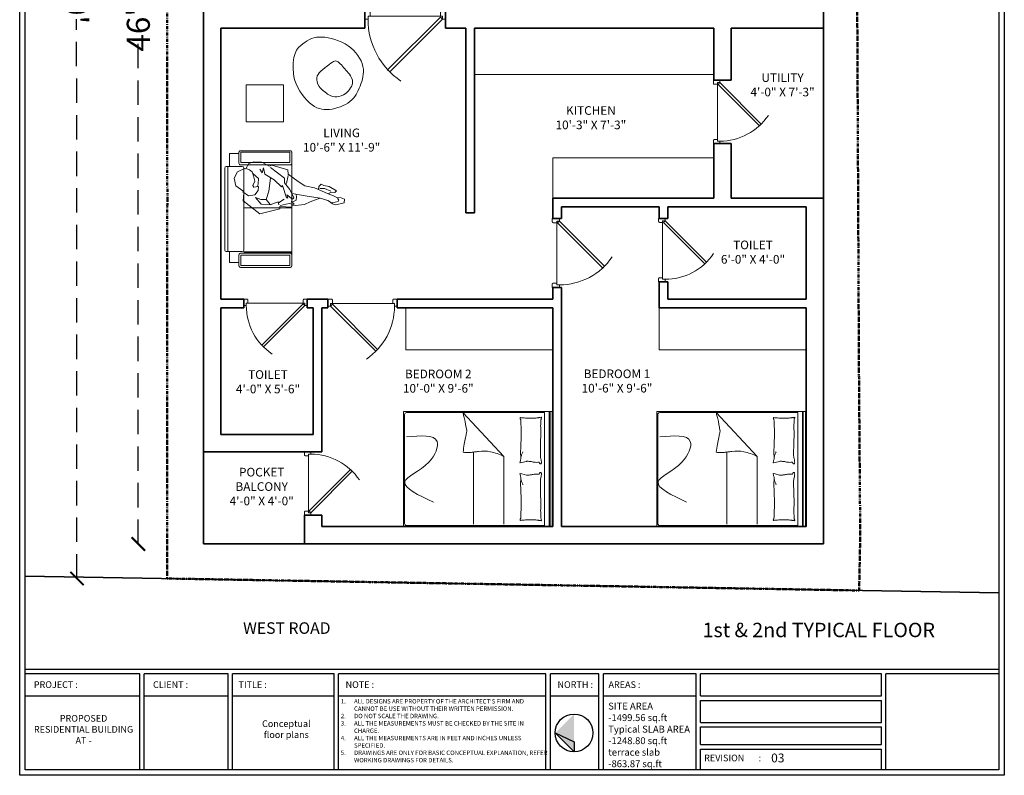
# Model space of a CAD drawing. Units: inches. Extents: x -16911 to -9621, y -48626 to -46270.
# Tile 2 of 20: x -16311 to -15799, y -47065 to -46672. Entities that reach past the tile are written whole.
import ezdxf

# ---------------------------------------------------------------- set-up
doc = ezdxf.new("R2010")
doc.units = ezdxf.units.IN
for name, pattern in [('DASHDOT', [1, 0.5, -0.25, 0, -0.25]), ('DASHED', [19.05, 12.7, -6.35]), ('DOT2', [3.175, 0, -3.175])]:
    doc.linetypes.add(name, pattern=pattern)
for name, color, linetype, lineweight in [('A-ANNO-DIMS', 2, 'Continuous', 13), ('A-ANNO-TEXT', 7, 'Continuous', 18), ('A-ANNO-TTLB', 7, 'Continuous', 25), ('A-AREA-IDEN', 3, 'Continuous', 18), ('A-DOOR', 4, 'Continuous', 18), ('A-FURN', 8, 'Continuous', 13), ('A-WALL', 7, 'Continuous', 35), ('C-PROP', 6, 'DASHDOT', 50), ('DOOR', 143, 'Continuous', 9), ('furniture', 35, 'Continuous', 15), ('Man', 8, 'Continuous', 5)]:
    doc.layers.add(name, color=color, linetype=linetype, lineweight=lineweight)
doc.styles.add('style9', font='swisscl.ttf', dxfattribs={"height": 12})
doc.dimstyles.new('Dim9', dxfattribs={"dimtxt": 10, "dimasz": 0.199219, "dimexe": 1, "dimexo": 0.5, "dimgap": 1, "dimtad": 0, "dimdec": 1, "dimzin": 0, "dimdsep": 46, "dimlunit": 4, "dimtxsty": 'style9', "dimblk": 'ARCHTICK', "dimcen": 0.09, "dimclrd": 256, "dimclrt": 256, "dimadec": 0, "dimazin": 0, "dimtfac": 1, "dimtdec": 1, "dimtix": 1, "dimtofl": 0, "dimtmove": 1, "dimatfit": 3, "dimfxl": 9, "dimtolj": 1, "dimtzin": 0, "dimlwd": -1, "dimarcsym": 0})

# ---------------------------------------------------------------- blocks, each defined once
blk = doc.blocks.new('Bipman02')
blk.add_lwpolyline([(0.5871, -0.067), (0.6175, -0.0496), (0.6523, -0.0539), (0.6697, -0.0376), (0.5958, 0.0069), (0.5437, 0.0156), (0.5164, 0.0297), (0.4959, 0.0069), (0.4915, -0.0235), (0.4524, -0.0061), (0.3568, 0.0113), (0.2917, 0.0548), (0.1917, 0.1287), (0.1874, 0.1722), (0.031, 0.2156), (0.0049, 0.2069), (-0.0689, 0.2461), (-0.1471, 0.2504), (-0.1949, 0.233), (-0.2253, 0.1808), (-0.2384, 0.1852), (-0.3079, 0.1504), (-0.3426, 0.0895), (-0.3253, 0.0113), (-0.2558, -0.0365), (-0.2471, -0.0583), (-0.2514, -0.1365), (-0.0863, -0.2626), (0.1092, -0.2148), (0.1092, -0.193), (0.2265, -0.1974), (0.2308, -0.1844), (0.3525, -0.1713), (0.409, -0.1452), (0.4872, -0.1148), (0.5089, -0.1104), (0.5828, -0.1322), (0.6088, -0.1496), (0.6295, -0.1636), (0.661, -0.1757), (0.7435, -0.1539), (0.7478, -0.1191), (0.7143, -0.1051), (0.674, -0.1017), (0.6392, -0.0844)], close=True)
for points in [[(-0.2558, -0.0452), (-0.1993, -0.0844), (-0.1385, -0.0757), (-0.1037, -0.0322), (-0.0994, 0.0069), (-0.1471, -0.0018), (-0.1558, 0.0156), (-0.1385, 0.0591), (-0.1515, 0.1113), (-0.1645, 0.1504), (-0.1906, 0.1722), (-0.2167, 0.1808)], [(-0.1558, 0.133), (-0.0994, 0.0852), (-0.1037, 0.033), (-0.1124, 0.0069)], [(-0.0863, 0.1765), (-0.0646, 0.1417), (-0.0516, 0.1895), (-0.0385, 0.1287), (0.0527, 0.0722), (0.1266, 0.0026), (0.1353, 0.0156), (0.1744, -0.1061), (0.1874, -0.1104), (0.1787, -0.0757), (0.2352, -0.1191), (0.2482, -0.1061), (0.2091, -0.0235), (0.157, 0.0417), (0.157, 0.0895), (0.018, 0.1939)], [(0.1917, 0.1156), (0.1744, 0.0374)], [(0.018, 0.0895), (0.0006, -0.0409), (-0.0255, -0.1235), (-0.0776, -0.1235), (-0.1298, -0.1017), (-0.0733, -0.167), (0.0136, -0.1757), (0.0918, -0.1452), (0.1005, -0.1757)], [(0.2699, -0.0757), (0.2743, -0.0974), (0.2699, -0.1278), (0.2439, -0.1409), (0.2222, -0.1452), (0.2482, -0.1626), (0.2482, -0.1713), (0.2004, -0.1626), (0.1135, -0.18)], [(0.2308, -0.0626), (0.3612, -0.0844), (0.5089, -0.1095)], [(0.4915, -0.0235), (0.5871, -0.067)], [(0.5045, -0.0148), (0.5523, -0.0148), (0.6132, -0.0409)], [(-0.0255, -0.1235), (0.0136, -0.1713)], [(0.0962, -0.1539), (0.1526, -0.1191)], [(0.6783, -0.1104), (0.6914, -0.1278), (0.687, -0.1409), (0.6566, -0.1496), (0.6088, -0.1539)]]:
    blk.add_lwpolyline(points)
blk = doc.blocks.new('erertety')
at = {"layer": 'furniture', "ltscale": 0.2}
for p, q in [((-17662.13, -45230.66), (-17662.13, -45176.69)), ((-17693.83, -45223.2), (-17693.83, -45184.43)), ((-17685.49, -45183.68), (-17693.08, -45183.68)), ((-17684.74, -45223.2), (-17684.74, -45184.43)), ((-17684.74, -45203.31), (-17662.13, -45203.31)), ((-17685.49, -45223.95), (-17693.08, -45223.95)), ((-17691.58, -45223.95), (-17691.58, -45229.1)), ((-17684.74, -45223.99), (-17662.13, -45223.99)), ((-17684.74, -45224.55), (-17662.13, -45224.55)), ((-17684.74, -45224.55), (-17662.13, -45224.55)), ((-17691.58, -45229.1), (-17687.09, -45229.1))]:
    blk.add_line(p, q, dxfattribs=at)
for points in [[(-17662.13, -45182.17), (-17662.13, -45176.97, 0.414214), (-17662.87, -45176.22), (-17686.34, -45176.22, 0.414214), (-17687.09, -45176.97), (-17687.09, -45182.17, 0.414214), (-17686.34, -45182.91), (-17662.87, -45182.91, 0.414214)], [(-17662.13, -45225.47), (-17662.13, -45230.66, -0.414214), (-17662.87, -45231.41), (-17686.34, -45231.41, -0.414214), (-17687.09, -45230.66), (-17687.09, -45225.47, -0.414214), (-17686.34, -45224.72), (-17662.87, -45224.72, -0.414214)]]:
    blk.add_lwpolyline(points, format="xyb", close=True, dxfattribs=at)
for points in [[(-17663.01, -45181.75), (-17663.01, -45176.82), (-17686.21, -45176.82), (-17686.21, -45181.75)], [(-17692.4, -45183.68), (-17692.4, -45223.95), (-17692.4, -45223.95), (-17692.4, -45183.68)], [(-17663.01, -45225.6), (-17663.01, -45230.53), (-17686.21, -45230.53), (-17686.21, -45225.6)]]:
    blk.add_lwpolyline(points, close=True, dxfattribs=at)
blk.add_lwpolyline([(-17687.09, -45177.54), (-17691.58, -45177.54), (-17691.58, -45183.68)], dxfattribs=at)
for centre, start, end in [((-17693.08, -45184.43), 90, 180), ((-17685.49, -45184.43), 0, 90), ((-17693.08, -45223.2), 180, 270), ((-17685.49, -45223.2), 270, 0)]:
    blk.add_arc(centre, 0.748, start, end, dxfattribs=at)
at = {"layer": 'furniture', "ltscale": 0.2, "xscale": 47.90818138957024, "yscale": 47.90818138957024, "zscale": 47.90818138957024}
blk.add_blockref('Bipman02', (-17673, -45193.44, 0), dxfattribs=at)
blk = doc.blocks.new('rthrty')
at = {"layer": 'furniture'}
blk.add_open_spline([(-17650.3, -45154.53), (-17651.97, -45142.9), (-17645.3, -45136.31), (-17637.11, -45132.37), (-17620.71, -45137.17), (-17612.47, -45149.45), (-17615.73, -45159.71), (-17619.67, -45168.02), (-17632.28, -45172.65), (-17641.84, -45170.43), (-17649.5, -45159.42), (-17650.3, -45154.53)], degree=3, dxfattribs=at)
at = {"layer": 'Man'}
blk.add_open_spline([(-17632.99, -45149.02), (-17629.89, -45146.6), (-17628, -45145.12), (-17623.29, -45151.15), (-17618.06, -45156.77), (-17623.15, -45164.08), (-17628.28, -45165.32), (-17631.61, -45164.6), (-17638.01, -45159.61), (-17638.81, -45154.69), (-17636.9, -45151.81), (-17632.99, -45149.02), (-17632.99, -45149.02)], degree=3, dxfattribs=at)
blk = doc.blocks.new('hjuyuiuyk')
at = {"layer": 'furniture'}
for p, q in [((-19327.49, -39738.98), (-19327.49, -39737.31)), ((-19327.49, -39737.31), (-19267.49, -39737.31, 0)), ((-19327.49, -39746.54), (-19327.49, -39737.31)), ((-19267.49, -39738.5), (-19327.49, -39738.5, 0)), ((-19327.49, -39738.5, 0), (-19327.49, -39814.72, 0)), ((-19327.49, -39738.5), (-19327.49, -39814.72)), ((-19267.49, -39738.5, 0), (-19327.49, -39738.5)), ((-19267.49, -39738.98, 0), (-19327.49, -39738.98)), ((-19267.49, -39737.31, 0), (-19267.49, -39738.98, 0)), ((-19267.49, -39746.54, 0), (-19267.49, -39737.31, 0)), ((-19267.49, -39814.72), (-19267.49, -39738.5)), ((-19267.49, -39814.72, 0), (-19267.49, -39738.5, 0)), ((-19268.1, -39741.33), (-19326.9, -39741.33)), ((-19326.9, -39741.33), (-19326.9, -39813.21)), ((-19268.1, -39813.21), (-19268.1, -39741.33)), ((-19300.88, -39753.22, 0), (-19301.49, -39750.81, 0)), ((-19300.67, -39754.09, 0), (-19300.88, -39753.22, 0)), ((-19295.19, -39754.09, 0), (-19294.97, -39753.22, 0)), ((-19294.97, -39753.22, 0), (-19294.37, -39750.81, 0)), ((-19304.07, -39762.52), (-19326.9, -39783.91)), ((-19304.07, -39762.52), (-19268.82, -39762.52)), ((-19268.82, -39778.34), (-19306.29, -39778.34)), ((-19326.9, -39813.21), (-19326.9, -39783.91)), ((-19327.49, -39814.72, 0), (-19267.49, -39814.72)), ((-19327.49, -39814.72), (-19267.49, -39814.72, 0)), ((-19269.1, -39814.21), (-19325.9, -39814.21)), ((-19325.9, -39814.21), (-19269.1, -39814.21))]:
    blk.add_line(p, q, dxfattribs=at)
for centre, radius, start, end in [((-19324.36, -39743.07, 0), 0.0997, 111.7883, 160.436), ((-19324.39, -39743.06, 0), 0.0676, 160.436, 281.8931), ((-19324.12, -39743.66, 0), 0.732, 94.3025, 111.7883), ((-19324.35, -39743.25, 0), 0.125, 21.9904, 101.8931), ((-19323.34, -39743.89, 0), 0.956, 158.579, 188.1335), ((-19317.18, -39743.01, 0), 7.17, 188.1335, 192.1095), ((-19324.65, -39743.37, 0), 0.455, 338.579, 21.9904), ((-19329.85, -39745.73, 0), 5.78, 7.6809, 12.1095), ((-19324.11, -39743.77, 0), 0.842, 59.3487, 94.3025), ((-19322.88, -39741.69, 0), 1.57, 239.3487, 264.7408), ((-19319.6, -39692.5, 0), 50.87, 266.1399, 268.6002), ((-19319.84, -39713.09, 0), 30.28, 268.0921, 271.2808), ((-19320.24, -39695.07, 0), 48.31, 271.2808, 273.4034), ((-19316.15, -39763.89, 0), 20.63, 90.1553, 93.4034), ((-19316.09, -39783.15, 0), 39.89, 86.9902, 90.1553), ((-19305.86, -39588.51, 0), 155.02, 266.9902, 268.5957), ((-19305.42, -39570.46, 0), 173.07, 268.5957, 270), ((-19305.42, -39718.38, 0), 25.15, 270, 273.6841), ((-19304.03, -39739.9, 0), 3.58, 273.6841, 287.1951), ((-19300.46, -39751.46, 0), 8.51, 98.4372, 107.1951), ((-19301.02, -39747.69, 0), 4.7, 90, 98.4372), ((-19301.12, -39743.14, 0), 0.997, 274.4002, 333.4195), ((-19315.3, -39745.68, 0), 14.34, 360, 6.2324), ((-19301.02, -39745.63, 0), 2.64, 78.7276, 90), ((-19300.58, -39743.42, 0), 0.383, 333.4195, 78.7276), ((-19295.28, -39743.42, 0), 0.383, 101.2724, 206.5805), ((-19294.73, -39743.14, 0), 0.997, 206.5805, 265.5998), ((-19294.84, -39745.63, 0), 2.64, 90, 101.2724), ((-19280.55, -39745.68, 0), 14.34, 173.7676, 180), ((-19294.84, -39747.69, 0), 4.7, 81.5628, 90), ((-19295.39, -39751.46, 0), 8.51, 72.8049, 81.5628), ((-19291.82, -39739.9, 0), 3.58, 252.8049, 266.3159), ((-19290.43, -39718.38, 0), 25.15, 266.3159, 270), ((-19290.43, -39570.46, 0), 173.07, 270, 271.4043), ((-19289.99, -39588.51, 0), 155.02, 271.4043, 273.0098), ((-19279.76, -39783.15, 0), 39.89, 89.8447, 93.0098), ((-19279.7, -39763.89, 0), 20.63, 86.5966, 89.8447), ((-19275.61, -39695.07, 0), 48.31, 266.5966, 268.7192), ((-19276.02, -39713.09, 0), 30.28, 268.7192, 271.9079), ((-19276.73, -39645.13, 0), 98.25, 271.0069, 272.7772), ((-19272.12, -39741.69, 0), 1.57, 275.2592, 300.6513), ((-19270.89, -39743.77, 0), 0.842, 85.6975, 120.6513), ((-19265.15, -39745.73, 0), 5.78, 167.8905, 172.3191), ((-19270.88, -39743.66, 0), 0.732, 68.2117, 85.6975), ((-19270.35, -39743.37, 0), 0.455, 158.0096, 201.421), ((-19277.82, -39743.01, 0), 7.17, 347.8905, 351.8665), ((-19270.65, -39743.25, 0), 0.125, 78.1069, 158.0096), ((-19271.66, -39743.89, 0), 0.956, 351.8665, 21.421), ((-19270.61, -39743.06, 0), 0.0676, 258.1069, 19.564), ((-19270.64, -39743.07, 0), 0.0997, 19.564, 68.2117), ((-19350.51, -39748.51, 0), 26.62, 3.3687, 7.6809), ((-19720.99, -39728.47, 0), 397.61, 356.4951, 356.945), ((-19363.7, -39747.54, 0), 39.81, 356.945, 358.3669), ((-19343.69, -39748.11, 0), 19.79, 358.3669, 3.3687), ((-19282.35, -39751.13, 0), 19.21, 171.9949, 177.3351), ((-19292.22, -39749.75, 0), 9.25, 167.8016, 171.9949), ((-19326.4, -39742.36, 0), 25.72, 347.8016, 350.3156), ((-19306.91, -39745.68, 0), 5.95, 350.3156, 360), ((-19288.94, -39745.68, 0), 5.95, 180, 189.6844), ((-19269.45, -39742.36, 0), 25.72, 189.6844, 192.1984), ((-19303.63, -39749.75, 0), 9.25, 8.0051, 12.1984), ((-19313.5, -39751.13, 0), 19.21, 2.6649, 8.0051), ((-19251.31, -39748.11, 0), 19.79, 176.6313, 181.6331), ((-19231.3, -39747.54, 0), 39.81, 181.6331, 183.055), ((-19244.49, -39748.51, 0), 26.62, 172.3191, 176.6313), ((-18874.01, -39728.47, 0), 397.61, 183.055, 183.5049), ((-19323.69, -39753.93, 0), 0.564, 170.0016, 196.6978), ((-19333.47, -39752.21, 0), 9.37, 350.0016, 356.4951), ((-19324.19, -39754.08, 0), 0.0385, 196.6978, 277.1204), ((-19324.51, -39751.59, 0), 2.55, 277.1204, 286.2212), ((-19324.42, -39751.9, 0), 2.23, 286.2212, 297.4439), ((-19322.81, -39754.99, 0), 1.25, 102.448, 117.4439), ((-19322.32, -39757.22, 0), 3.54, 93.574, 102.448), ((-19318.44, -39837.61, 0), 84.03, 90.9755, 92.7955), ((-19315.55, -39952.16, 0), 198.61, 89.4461, 91.2473), ((-19314.9, -39885.06, 0), 131.51, 87.2326, 89.4461), ((-19310.57, -39795.48, 0), 41.81, 85.4012, 87.2326), ((-19304.32, -39717.78, 0), 36.14, 265.4012, 267.3712), ((-19297.32, -39733.09, 0), 21.54, 244.6889, 246.5156), ((-19305.66, -39747.05, 0), 6.83, 267.3712, 281.4827), ((-19297.32, -39733.09, 0), 21.54, 246.5156, 248.3423), ((-19297.32, -39733.09, 0), 21.54, 248.3423, 250.572), ((-19297.32, -39733.09, 0), 21.54, 250.572, 252.8018), ((-19303.46, -39757.91, 0), 4.25, 83.5659, 101.4827), ((-19303.37, -39757.16, 0), 3.49, 72.6136, 83.5659), ((-19300.33, -39747.43, 0), 6.7, 252.6136, 260.5159), ((-19299.57, -39750.33, 0), 1.97, 177.3351, 194.0452), ((-19300.13, -39746.25, 0), 7.9, 260.5159, 265.9171), ((-19300.69, -39754.1, 0), 0.0267, 265.9171, 14.0449), ((-19295.16, -39754.1, 0), 0.0267, 165.9551, 274.0829), ((-19295.72, -39746.25, 0), 7.9, 274.0829, 279.4841), ((-19295.52, -39747.43, 0), 6.7, 279.4841, 287.3864), ((-19296.28, -39750.33, 0), 1.97, 345.9548, 2.6649), ((-19292.48, -39757.16, 0), 3.49, 96.4341, 107.3864), ((-19292.39, -39757.91, 0), 4.25, 78.5173, 96.4341), ((-19298.54, -39733.09, 0), 21.54, 287.1982, 289.428), ((-19290.19, -39747.05, 0), 6.83, 258.5173, 272.6288), ((-19298.54, -39733.09, 0), 21.54, 289.428, 291.6577), ((-19298.54, -39733.09, 0), 21.54, 291.6577, 293.4844), ((-19298.54, -39733.09, 0), 21.54, 293.4844, 295.3111), ((-19291.53, -39717.78, 0), 36.14, 272.6288, 274.5988), ((-19285.28, -39795.48, 0), 41.81, 92.7674, 94.5988), ((-19280.95, -39885.06, 0), 131.51, 90.5539, 92.7674), ((-19280.3, -39952.16, 0), 198.61, 88.7527, 90.5539), ((-19277.1, -39805.01, 0), 51.42, 86.426, 88.7527), ((-19274.68, -39799.75, 0), 46.07, 86.5575, 89.0171), ((-19272.19, -39754.99, 0), 1.25, 62.5561, 77.552), ((-19270.58, -39751.9, 0), 2.23, 242.5561, 253.7788), ((-19270.49, -39751.59, 0), 2.55, 253.7788, 262.8796), ((-19261.53, -39752.21, 0), 9.37, 183.5049, 189.9984), ((-19270.81, -39754.08, 0), 0.0385, 262.8796, 343.3022), ((-19271.31, -39753.93, 0), 0.564, 343.3022, 9.9984), ((-19279.47, -39774.89), 27.53, 153.3084, 168.7423), ((-19287.94, -39773.2), 18.89, 168.7423, 187.3994), ((-19242.78, -39767.34), 64.43, 187.3994, 189.2719), ((-19333.07, -39782.08), 27.05, 6.3817, 9.2719), ((-19321.79, -39780.82), 15.7, 359.2313, 6.3817), ((-19306.77, -39846.83), 66.07, 105.9352, 107.7364), ((-19318.41, -39806.06), 23.67, 102.9255, 105.9352), ((-19287.64, -39956.87), 177.57, 99.7243, 101.7196), ((-19317.24, -39783.9), 2.09, 82.2696, 100.7276), ((-19317.9, -39788.76), 6.99, 76.8096, 82.2696), ((-19295.64, -39693.77), 90.57, 256.8096, 258.3259), ((-19295.11, -39691.23), 93.17, 258.3259, 260.505), ((-19288.03, -39648.9), 136.08, 260.505, 262.308), ((-19336.71, -39780.62), 30.63, 354.1141, 359.2313), ((-19325.9, -39813.21), 1, 180, 270), ((-19269.1, -39813.21), 1, 270, 0)]:
    blk.add_arc(centre, radius, start, end, dxfattribs=at)
blk.add_open_spline([(-19280.24, -39799.21), (-19283.87, -39806.94), (-19290.73, -39821.55), (-19298.08, -39801.09), (-19315.85, -39793.47), (-19314.86, -39805.92), (-19314.29, -39813.13)], degree=3, knots=[0, 0, 0, 0, 18.167809, 34.338432, 45.972904, 61.997799, 61.997799, 61.997799, 61.997799], dxfattribs=at)
blk = doc.blocks.new('A$C1C9D3E54')
at = {"layer": 'DOOR'}
blk.add_line((18676.53, 5780.72), (18710.53, 5780.72), dxfattribs=at)
blk.add_lwpolyline([(18685.01, 5806.62), (18710.47, 5781.16), (18711.53, 5782.22), (18686.07, 5807.68), (18685.01, 5806.62)], dxfattribs=at)
blk.add_lwpolyline([(18674.03, 5778.22), (18676.03, 5778.22), (18674.03, 5778.22), (18674.03, 5782.22), (18675.53, 5782.22), (18675.53, 5780.72), (18676.53, 5780.72), (18676.53, 5778.72), (18676.41, 5778.72), (18676.41, 5778.6, -0.414214), (18676.16, 5778.35), (18676.03, 5778.35), (18676.03, 5778.22)], format="xyb", dxfattribs=at)
blk.add_lwpolyline([(18713.03, 5782.22), (18711.53, 5782.22), (18711.53, 5780.72), (18710.53, 5780.72), (18710.53, 5778.72), (18710.66, 5778.72), (18710.66, 5778.6, 0.414214), (18710.91, 5778.35), (18711.03, 5778.35), (18711.03, 5778.22), (18713.03, 5778.22), (18711.03, 5778.22), (18713.03, 5778.22), (18713.03, 5782.22)], format="xyb", close=True, dxfattribs=at)
blk.add_arc((18711.53, 5782.22), 36, 124.0336, 180, dxfattribs=at)
blk = doc.blocks.new('_ArchTick')
at = {"color": 0, "linetype": 'ByBlock', "const_width": 0.15}
blk.add_lwpolyline([(-0.5, -0.5), (0.5, 0.5)], dxfattribs=at)
blk = doc.blocks.new('*D58')
at = {"layer": 'A-ANNO-DIMS', "color": 0, "linetype": 'DOT2', "lineweight": -2, "transparency": 16777216}
for p, q in [((-16281.81, -46362.82), (-16283, -46362.82)), ((-16281.44, -46962.82), (-16282.63, -46962.82))]:
    blk.add_line(p, q, dxfattribs=at)
at = {"layer": 'A-ANNO-DIMS', "color": 0, "linetype": 'DASHED', "lineweight": 25, "transparency": 16777216}
for p, q in [((-16282, -46362.82), (-16281.82, -46653.98)), ((-16281.63, -46962.82), (-16281.81, -46671.67))]:
    blk.add_line(p, q, dxfattribs=at)
at = {"layer": 'Defpoints', "color": 0, "transparency": 16777216}
for p in [(-16282, -46362.82), (-16263.18, -46362.81), (-16262.82, -46962.81)]:
    blk.add_point(p, dxfattribs=at)
at = {"layer": 'A-ANNO-DIMS', "color": 0, "lineweight": 25, "transparency": 16777216, "xscale": 7, "yscale": 7, "zscale": 7}
for p, rotation in [((-16282, -46362.82), 90.0346840750536), ((-16281.63, -46962.82), 270.0346840750536)]:
    blk.add_blockref('_ArchTick', p, dxfattribs=dict(at, rotation=rotation))
at = {"layer": 'A-ANNO-DIMS', "color": 0, "transparency": 16777216, "insert": (-16281.81, -46662.82), "char_height": 12, "attachment_point": 5, "rotation": 270.0347, "style": 'style9'}
blk.add_mtext("\\A1;50'", dxfattribs=at)
blk = doc.blocks.new('*D60')
at = {"layer": 'A-ANNO-DIMS', "color": 0, "linetype": 'DOT2', "lineweight": -2, "transparency": 16777216}
for p, q in [((-16249.52, -46386.86), (-16250.71, -46386.86)), ((-16249.52, -46944.81), (-16250.71, -46944.81))]:
    blk.add_line(p, q, dxfattribs=at)
at = {"layer": 'A-ANNO-DIMS', "color": 0, "linetype": 'DASHED', "lineweight": 25, "transparency": 16777216}
for p, q in [((-16249.71, -46386.86), (-16249.71, -46648.2)), ((-16249.71, -46944.81), (-16249.71, -46683.47))]:
    blk.add_line(p, q, dxfattribs=at)
at = {"layer": 'Defpoints', "color": 0, "transparency": 16777216}
for p in [(-16215.78, -46386.86), (-16249.71, -46944.81), (-16215.78, -46944.81)]:
    blk.add_point(p, dxfattribs=at)
at = {"layer": 'A-ANNO-DIMS', "color": 0, "lineweight": 25, "transparency": 16777216, "xscale": 7, "yscale": 7, "zscale": 7}
for p, rotation in [((-16249.71, -46386.86), 90), ((-16249.71, -46944.81), 270)]:
    blk.add_blockref('_ArchTick', p, dxfattribs=dict(at, rotation=rotation))
at = {"layer": 'A-ANNO-DIMS', "color": 0, "transparency": 16777216, "insert": (-16249.71, -46665.83), "char_height": 12, "attachment_point": 5, "rotation": 90, "style": 'style9'}
blk.add_mtext('\\A1;46\'-6"', dxfattribs=at)
blk = doc.blocks.new('TITLE-BLOCK-A3')
blk.add_hatch(color=256).paths.add_polyline_path([(-16032.81, -47043.2), (-16022.97, -47033.35), (-16022.97, -47053.05)])
for p, q in [((-16311.44, -47065.27), (-16311.44, -46330.13)), ((-16308.66, -47062.49), (-16308.66, -46332.91)), ((-15801.86, -46332.91), (-15801.86, -47062.49)), ((-15799.07, -46330.13), (-15799.07, -47065.27)), ((-15801.86, -47010.14), (-16308.66, -47010.14)), ((-16248.93, -47012.43), (-16308.66, -47012.43)), ((-16248.93, -47062.49), (-16248.93, -47012.43)), ((-16202.98, -47012.43), (-16246.63, -47012.43)), ((-16246.63, -47062.49), (-16246.63, -47012.43)), ((-16202.98, -47062.49), (-16202.98, -47012.43)), ((-16147.85, -47012.43), (-16200.68, -47012.43)), ((-16200.68, -47062.49), (-16200.68, -47012.43)), ((-16147.85, -47062.49), (-16147.85, -47012.43)), ((-16037.57, -47012.43), (-16145.55, -47012.43)), ((-16145.55, -47062.49), (-16145.55, -47012.43)), ((-16037.57, -47062.49), (-16037.57, -47012.43)), ((-16010.01, -47012.43), (-16035.28, -47012.43)), ((-16035.28, -47062.49), (-16035.28, -47012.43)), ((-16010.01, -47062.49), (-16010.01, -47012.43)), ((-15959.47, -47012.43), (-16007.71, -47012.43)), ((-16007.71, -47062.49), (-16007.71, -47012.43)), ((-15959.47, -47062.49), (-15959.47, -47012.43)), ((-15862.98, -47012.43), (-15957.17, -47012.43)), ((-15957.17, -47023.95), (-15957.17, -47012.43)), ((-15862.98, -47023.95), (-15862.98, -47012.43)), ((-15801.86, -47012.43), (-15860.68, -47012.43)), ((-15860.68, -47062.49), (-15860.68, -47012.43)), ((-16308.66, -47023.95), (-16248.93, -47023.95)), ((-16246.63, -47023.95), (-16202.98, -47023.95)), ((-16200.68, -47023.95), (-16147.85, -47023.95)), ((-16145.55, -47023.95), (-16037.57, -47023.95)), ((-16035.28, -47023.95), (-16010.01, -47023.95)), ((-16007.71, -47023.95), (-15959.47, -47023.95)), ((-15957.17, -47023.95), (-15862.98, -47023.95)), ((-15957.17, -47037.77), (-15957.17, -47026.25)), ((-15957.17, -47026.25), (-15862.98, -47026.25)), ((-15862.98, -47037.77), (-15862.98, -47026.25)), ((-15957.17, -47037.77), (-15862.98, -47037.77)), ((-15957.17, -47049.29), (-15957.17, -47040.07)), ((-15957.17, -47040.07), (-15862.98, -47040.07)), ((-15862.98, -47049.29), (-15862.98, -47040.07)), ((-15957.17, -47049.29), (-15862.98, -47049.29)), ((-15957.17, -47062.49), (-15957.17, -47051.59)), ((-15862.98, -47062.49), (-15862.98, -47051.59)), ((-15799.07, -47065.27), (-16311.44, -47065.27)), ((-15801.86, -47062.49), (-16308.66, -47062.49))]:
    blk.add_line(p, q)
blk.add_lwpolyline([(-16032.81, -47043.2), (-16022.97, -47047.92), (-16022.97, -47053.05), (-16032.81, -47043.2)])
blk.add_circle((-16022.97, -47043.2), 9.85)

msp = doc.modelspace()

# ---------------------------------------------------------------- linework, layer by layer
at = {"layer": 'A-ANNO-TTLB'}
msp.add_line((-15957.168, -47051.592), (-15862.978, -47051.592), dxfattribs=at)
at = {"layer": 'A-FURN', "ltscale": 0.2}
for p, q in [((-15950.233, -46700.355), (-16074.783, -46700.355)), ((-15950.233, -46743.809), (-16034.033, -46743.809)), ((-16034.033, -46764.809), (-16034.033, -46743.809)), ((-16110.533, -46821.809, 0), (-16110.533, -46843.809, 0)), ((-15978.733, -46821.809), (-15978.733, -46843.809)), ((-16034.033, -46843.809), (-16110.533, -46843.809)), ((-15978.733, -46843.809), (-15902.233, -46843.809))]:
    msp.add_line(p, q, dxfattribs=at)
at = {"layer": 'A-FURN'}
msp.add_lwpolyline([(-16174.187, -46705.751), (-16193.547, -46705.751), (-16193.547, -46725.111), (-16174.187, -46725.111)], close=True, dxfattribs=at)
at = {"layer": 'A-WALL'}
for p, q in [((-16215.783, -46896.809), (-16215.783, -46434.855)), ((-15893.233, -46469.355), (-15893.233, -46676.355)), ((-16131.783, -46676.355), (-16131.783, -46667.355)), ((-16089.783, -46676.355), (-16089.783, -46667.355)), ((-16206.783, -46817.309), (-16206.783, -46676.355)), ((-16131.783, -46676.355), (-16206.783, -46676.355)), ((-16079.283, -46676.355), (-16089.783, -46676.355)), ((-16079.283, -46676.355), (-16079.283, -46772.355)), ((-15950.233, -46676.355), (-16074.783, -46676.355)), ((-16074.783, -46676.355), (-16074.783, -46772.355)), ((-15950.233, -46676.355), (-15950.233, -46703.355)), ((-15893.233, -46676.355), (-15941.233, -46676.355)), ((-15941.233, -46676.355), (-15941.233, -46703.355)), ((-15893.233, -46676.355), (-15893.233, -46764.809)), ((-15950.233, -46703.355), (-15941.233, -46703.355)), ((-15950.233, -46736.355), (-15950.233, -46764.809)), ((-15950.233, -46736.355), (-15941.233, -46736.355)), ((-15941.233, -46736.355), (-15941.233, -46764.809)), ((-16034.033, -46775.309), (-16034.033, -46764.809)), ((-16034.033, -46764.809), (-15950.233, -46764.809)), ((-15941.233, -46764.809), (-15893.233, -46764.809)), ((-15893.233, -46764.809), (-15893.233, -46944.809)), ((-16074.783, -46772.355), (-16079.283, -46772.355)), ((-16029.533, -46775.309), (-16029.533, -46769.309)), ((-16029.533, -46769.309), (-15978.733, -46769.309)), ((-15978.733, -46769.309), (-15978.733, -46775.309)), ((-15974.233, -46769.309), (-15974.233, -46775.309)), ((-15974.233, -46769.309), (-15902.233, -46769.309)), ((-15902.233, -46769.309), (-15902.233, -46817.309)), ((-16034.033, -46775.309), (-16029.533, -46775.309)), ((-15978.733, -46775.309), (-15974.233, -46775.309)), ((-15978.733, -46808.309), (-15978.733, -46821.809)), ((-15978.733, -46808.309), (-15974.233, -46808.309)), ((-15974.233, -46808.309), (-15974.233, -46817.309)), ((-16034.033, -46817.309), (-16034.033, -46811.309)), ((-16034.033, -46811.309), (-16029.533, -46811.309)), ((-16029.533, -46935.809), (-16029.533, -46811.309)), ((-16206.783, -46817.309), (-16194.783, -46817.309)), ((-16194.783, -46817.309), (-16194.783, -46821.809)), ((-16161.783, -46817.309), (-16151.033, -46817.309)), ((-16161.783, -46817.309), (-16161.783, -46821.809)), ((-16151.033, -46821.809), (-16151.033, -46817.309)), ((-16115.033, -46817.309), (-16034.033, -46817.309)), ((-16115.033, -46821.809), (-16115.033, -46817.309)), ((-15974.233, -46817.309), (-15902.233, -46817.309)), ((-16206.783, -46887.809), (-16206.783, -46821.809)), ((-16206.783, -46821.809), (-16194.783, -46821.809)), ((-16161.783, -46821.809), (-16158.783, -46821.809)), ((-16158.783, -46887.809), (-16158.783, -46821.809)), ((-16154.283, -46896.809), (-16154.283, -46821.809)), ((-16154.283, -46821.809), (-16151.033, -46821.809)), ((-16115.033, -46821.809), (-16034.033, -46821.809)), ((-16034.033, -46935.809), (-16034.033, -46821.809)), ((-15978.733, -46821.809), (-15902.233, -46821.809)), ((-15902.233, -46821.809), (-15902.233, -46935.809)), ((-16206.783, -46887.809), (-16158.783, -46887.809)), ((-16215.783, -46944.809), (-16215.783, -46896.809)), ((-16215.783, -46896.809), (-16154.283, -46896.809)), ((-16163.283, -46944.809), (-16163.283, -46929.809)), ((-16163.283, -46929.809), (-16154.283, -46929.809)), ((-16154.283, -46935.809), (-16154.283, -46929.809)), ((-16154.283, -46935.809), (-16034.033, -46935.809)), ((-16029.533, -46935.809), (-15902.233, -46935.809)), ((-16215.783, -46944.809), (-16163.283, -46944.809)), ((-16163.283, -46944.809), (-15893.233, -46944.809)), ((-15801.856, -46970.292), (-16308.658, -46961.533))]:
    msp.add_line(p, q, dxfattribs=at)
at = {"layer": 'C-PROP'}
msp.add_lwpolyline([(-16234.783, -46962.809), (-15874.601, -46969.035), (-15874.04, -46940.446), (-15874.703, -46855.606), (-15875.869, -46609.511), (-15875.483, -46367.855), (-16235.146, -46362.811), (-16234.608, -46762.955)], close=True, dxfattribs=at)

# ---------------------------------------------------------------- block references
at = {"layer": 'A-ANNO-TTLB'}
msp.add_blockref('TITLE-BLOCK-A3', (0, 0), dxfattribs=at)
at = {"layer": 'A-DOOR'}
for p, xscale, yscale, zscale, rotation in [((-36242.277, -40444.653), -1.076923076922859, 1.076923076922859, 1.076923076922859, 180), ((-20839.75, -62537.458), -0.8461538461538624, 0.8461538461538624, 0.8461538461538624, 270), ((-21368.028, -64048.876), -0.9230769230769229, 0.9230769230769229, 0.9230769230769229, 270), ((-20868.25, -62609.412), -0.8461538461538624, 0.8461538461538624, 0.8461538461538624, 270), ((-31995.886, -41928.043), -0.8461538461538624, 0.8461538461538624, 0.8461538461538624, 180), ((1122.534, -41483.564), 0.9230769230769229, 0.9230769230769229, 0.9230769230769229, 180), ((-21052.549, -31095.706), 0.8461538461538624, 0.8461538461538624, 0.8461538461538624, 270)]:
    msp.add_blockref('A$C1C9D3E54', p, dxfattribs=dict(at, xscale=xscale, yscale=yscale, zscale=zscale, rotation=rotation))
at = {"layer": 'A-FURN'}
msp.add_blockref('rthrty', (1481.543, -1547.053), dxfattribs=at)
at = {"layer": 'A-FURN', "xscale": 1.1, "yscale": 1.1, "zscale": 1.1}
msp.add_blockref('erertety', (3258.451, 2953.75, 0), dxfattribs=at)
at = {"layer": 'A-FURN', "rotation": 270}
for p in [(23703.029, -66203.296), (23834.829, -66203.296, 0)]:
    msp.add_blockref('hjuyuiuyk', p, dxfattribs=at)

# ---------------------------------------------------------------- texts
at = {"layer": 'A-ANNO-TEXT', "ltscale": 10, "style": 'style9'}
for s, insert, char_height, width, attachment_point in [('\\A1;{\\fCentury Gothic|b0|i0|c0|p34;WEST ROAD}', (-16195.193, -46985.611), 6, 70.69764, 1), ('\\A1;{\\fCentury Gothic|b0|i0|c0|p34;1st & 2nd TYPICAL FLOOR}', (-15956.089, -46985.845), 7.5, 166.78033, 1), ('\\A1;\\pxql;{\\fCentury Gothic|b0|i0|c0|p34;PROJECT :}', (-16165.778, -47016.326), 3.44598, 138.32013, 3), ('\\A1;\\pxql;{\\fCentury Gothic|b0|i0|c0|p34;CLIENT :}', (-16087.669, -47016.326), 3.44598, 154.40134, 3), ('\\A1;\\pxql;{\\fCentury Gothic|b0|i0|c0|p34;TITLE :}', (-16059.24, -47016.326), 3.44598, 138.32013, 3), ('\\A1;\\pxql;{\\fCentury Gothic|b0|i0|c0|p34;NOTE :}', (-15973.671, -47016.326), 3.44598, 168.18525, 3), ('\\A1;\\pxql;{\\fCentury Gothic|b0|i0|c0|p34;NORTH :}', (-15863.4, -47016.326), 3.44598, 168.18525, 3), ('\\A1;\\pxql;{\\fCentury Gothic|b0|i0|c0|p34;AREAS :}', (-15866.711, -47016.326), 3.44598, 138.32013, 3), ("\\pxi-3,l4,ql,t4;{\\fArial|b0|i0|c0|p34;1.^IALL DESIGNS ARE PROPERTY OF THE ARCHITECT'S FIRM AND CANNOT BE USE WITHOUT THEIR WRITTEN PERMISSION.\\P2.^IDO NOT SCALE THE DRAWING.\\P3.^IALL THE MEASUREMENTS MUST BE CHECKED BY THE SITE IN CHARGE.\\P4.^IALL THE MEASUREMENTS ARE IN FEET AND INCHES UNLESS SPECIFIED.\\P5.^IDRAWINGS ARE ONLY FOR BASIC CONCEPTUAL EXPLANATION, REFER WORKING DRAWINGS FOR DETAILS.}", (-16036.219, -47025.582), 2.297317, 110.42201, 3), ('\\A1;{\\fCentury Gothic|b0|i0|c0|p34;SITE AREA\\P-1499.56 sq.ft\\PTypical SLAB AREA \\P-1248.80 sq.ft\\Pterrace slab \\P-863.87 sq.ft }', (-16005.181, -47061.046), 3.6, 46.67019, 7), ('\\A1;\\pxqc;{\\fCentury Gothic|b0|i0|c0|p34;PROPOSED RESIDENTIAL BUILDING AT -}', (-16251.087, -47033.885), 3.44598, 54.24005, 3), ('\\A1;\\pxqc;{\\fCentury Gothic|b0|i0|c0|p34;Conceptual\\Pfloor plans}', (-16158.709, -47036.671), 3.44598, 27.96068, 3), ('\\A1;\\pxql;{\\fCentury Gothic|b0|i0|c0|p34;REVISION       :     \\H1.33333x;03}', (-15816.939, -47053.939), 3.44598, 138.32013, 3)]:
    msp.add_mtext(s, dxfattribs=dict(at, insert=insert, char_height=char_height, width=width, attachment_point=attachment_point))
at = {"layer": 'A-AREA-IDEN', "ltscale": 10, "char_height": 4.5, "width": 42.823, "attachment_point": 1, "style": 'style9'}
for s, insert in [('\\A1;\\pxqc;{\\fCentury Gothic|b0|i0|c0|p34;UTILITY\\P4\'-0" X 7\'-3"}', (-15935.873, -46699.772)), ('\\A1;\\pxqc;{\\fCentury Gothic|b0|i0|c0|p34;KITCHEN\\P10\'-3" X 7\'-3"}', (-16035.607, -46716.893)), ('\\A1;\\pxqc;{\\fCentury Gothic|b0|i0|c0|p34;LIVING\\P10\'-6" X 11\'-9"}', (-16165.321, -46728.541)), ('\\A1;\\pxqc;{\\fCentury Gothic|b0|i0|c0|p34;TOILET\\P6\'-0" X 4\'-0"}', (-15951.259, -46786.873)), ('\\A1;\\pxqc;{\\fCentury Gothic|b0|i0|c0|p34;TOILET\\P4\'-0" X 5\'-6"}', (-16203.639, -46854.373)), ('\\A1;\\pxqc;{\\fCentury Gothic|b0|i0|c0|p34;BEDROOM 2\\P10\'-0" X 9\'-6"}', (-16115.03, -46854.047)), ('\\A1;\\pxqc;{\\fCentury Gothic|b0|i0|c0|p34;BEDROOM 1\\P10\'-6" X 9\'-6"}', (-16022.036, -46853.971)), ('\\A1;\\pxqc;{\\fCentury Gothic|b0|i0|c0|p34;POCKET BALCONY\\P4\'-0" X 4\'-0"}', (-16206.923, -46905.176))]:
    msp.add_mtext(s, dxfattribs=dict(at, insert=insert))

# ---------------------------------------------------------------- dimensions: what is measured, and where the dimension line sits
at = {"layer": 'A-ANNO-DIMS'}
dim = msp.add_aligned_dim(p1=(-16262.815, -46962.809), p2=(-16263.178, -46362.811), distance=18.817, dimstyle='Dim9', override={"dimtxt": 12, "dimasz": 7, "dimdec": 2, "dimclrd": 0, "dimclre": 0, "dimclrt": 0, "dimtdec": 2, "dimfxl": 0.1875, "dimfxlon": 1, "dimlwd": 25, "dimarcsym": 2}, dxfattribs=at)
dim.commit()
dim.dimension.update_dxf_attribs({"geometry": '*D58', "text_midpoint": (-16281.814, -46662.821)})
dim = msp.add_linear_dim(base=(-16249.711, -46944.809), p1=(-16215.783, -46386.855), p2=(-16215.783, -46944.809), angle=90, dimstyle='Dim9', override={"dimtxt": 12, "dimasz": 7, "dimdec": 2, "dimclrd": 0, "dimclre": 0, "dimclrt": 0, "dimtdec": 2, "dimfxl": 0.1875, "dimfxlon": 1, "dimlwd": 25, "dimarcsym": 2}, dxfattribs=at)
dim.commit()
dim.dimension.update_dxf_attribs({"geometry": '*D60', "text_midpoint": (-16249.711, -46665.832)})

doc.saveas('drawing.dxf')
